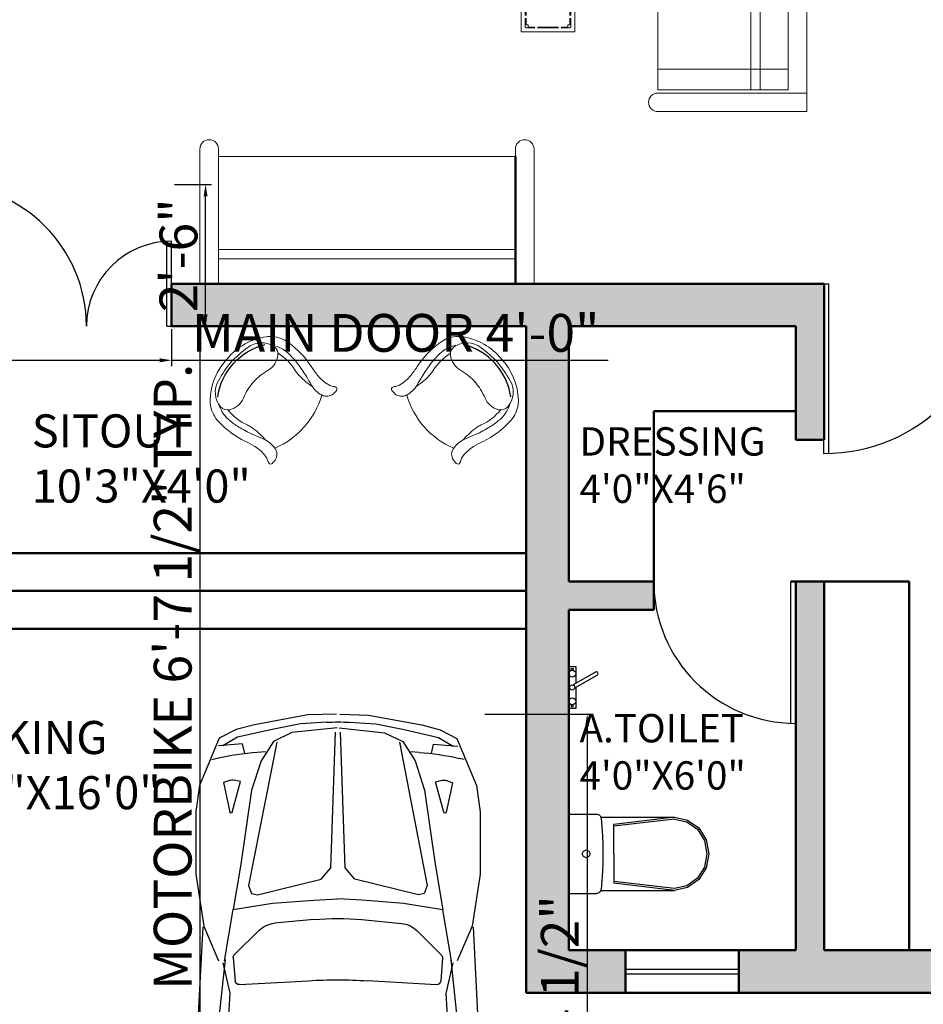
# Model space of a CAD drawing. Units: inches. Extents: x 3008 to 4088, y 1255 to 2137.
# Tile 5 of 30: x 3119 to 3310, y 1462 to 1670. Entities that reach past the tile are written whole.
import ezdxf

# ---------------------------------------------------------------- set-up
doc = ezdxf.new("R2010")
doc.units = ezdxf.units.IN
for name, color, linetype, lineweight in [('A-ANNO-DIMS', 2, 'Continuous', 18), ('A-AREA-IDEN', 7, 'Continuous', 18), ('A-DOOR', 4, 'Continuous', 25), ('A-FLOR-FIXT', 8, 'Continuous', 18), ('A-FURN', 8, 'Continuous', 18), ('A-GLAZ', 4, 'Continuous', 25), ('A-WALL', 7, 'Continuous', 50), ('A-WALL-PATT', 8, 'Continuous', 13), ('C-SITE-VEHC', 9, 'Continuous', 13)]:
    doc.layers.add(name, color=color, linetype=linetype, lineweight=lineweight)
for name, color, linetype in [('IFF-FURN-DETAIL', 250, 'Continuous'), ('L9012X$0', 2, 'Continuous'), ('SANTEH', 7, 'Continuous')]:
    doc.layers.add(name, color=color, linetype=linetype)
doc.styles.get("Standard").update_dxf_attribs({"font": 'arial.ttf'})
doc.dimstyles.new('ISO-25', dxfattribs={"dimtxt": 8, "dimasz": 2.5, "dimexe": 1.25, "dimexo": 0.625, "dimtad": 1, "dimdec": 1, "dimlunit": 3, "dimtxsty": 'Standard', "dimcen": 2.5, "dimadec": 0, "dimazin": 0, "dimtfac": 1, "dimtdec": 1, "dimtmove": 0, "dimatfit": 3, "dimfxl": 1, "dimarcsym": 0})

# ---------------------------------------------------------------- blocks, each defined once
blk = doc.blocks.new('MD')
for p, q in [((1902.58, 1512.86), (1902.58, 1482.86)), ((1903.58, 1512.86), (1903.58, 1482.86)), ((1949.58, 1482.86), (1949.58, 1500.86)), ((1950.58, 1482.86), (1950.58, 1500.86)), ((1902.58, 1482.86), (1903.58, 1482.86)), ((1949.58, 1482.86), (1950.58, 1482.86))]:
    blk.add_line(p, q)
for centre, radius, start, end in [((1902.58, 1482.86), 30, 0, 90), ((1950.58, 1482.86), 18, 90, 180)]:
    blk.add_arc(centre, radius, start, end)
blk = doc.blocks.new('A1099DC')
at = {"color": 0, "linetype": 'ByBlock'}
for p, q in [((1279.298465, 804.448389), (2201.430588, 851.890505)), ((2602.736326, 846.078152), (3356.693814, 785.353187)), ((3488.458929, 772.663345), (3732.658862, 759.86454)), ((272.228253, 749.073842), (265.114727, 718.465169)), ((1475.52921, 670.226262), (2282.402739, 758.004075)), ((2519.280414, 756.817792), (3387.476361, 653.818028)), ((2851.341839, 715.213377), (3126.60716, 755.701993)), ((139.051458, 595.027331), (190.951238, 683.213377)), ((179.200345, 564.515703), (190.951238, 709.631982)), ((398.733388, 644.315148), (411.280494, 678.748261)), ((411.280494, 678.748261), (588.616917, 641.417897)), ((1482.852352, 674.283145), (1175.286956, 622.180789)), ((1494.603245, 682.841284), (1678.210958, 641.166865)), ((1678.210958, 641.166865), (2462.684993, 690.847736)), ((2656.476214, 692.831247), (3376.704709, 662.004075)), ((3376.704709, 662.004075), (3510.708679, 626.736433)), ((3909.27561, 688.812956), (3837.725727, 693.401722)), ((3867.794139, 700.329656), (3900.059395, 686.767505)), ((3921.162781, 527.618662), (3921.162781, 676.138994)), ((3925.383812, 676.122818), (3955.306409, 663.545364)), ((92.537504, 388.14361), (139.051458, 595.027331)), ((405.405047, 577.538958), (396.874865, 615.894428)), ((589.014326, 626.599587), (405.405047, 577.538958)), ((1300.814287, 466.658131), (1445.712032, 613.104998)), ((1465.665584, 620.56924), (1602.893878, 610.287296)), ((236.043912, 551.980927), (179.200345, 564.515703)), ((1626.354615, 583.507504), (1602.652901, 169.222264)), ((3704.596898, 536.993674), (3795.675135, 473.385795)), ((229.117398, 477.634662), (225.714299, 427.957563)), ((1933.148906, 509.557888), (2330.980062, 522.200075)), ((3522.252709, 492.345257), (3666.066199, 475.644444)), ((3841.786866, 503.451367), (3910.58243, 515.096797)), ((3901.001848, 514.780764), (3957.150905, 375.772812)), ((1860.238743, -448.635916), (1859.369151, 433.397797)), ((2409.60024, 445.938054), (2410.49349, -460.09121)), ((3493.960271, 465.734554), (3507.923021, 209.166865)), ((3839.396146, 426.841284), (3888.358202, 417.538958)), ((3888.358202, 417.538958), (3983.199613, 359.957848)), ((57.774444, 216.608726), (92.537504, 388.14361)), ((1235.045743, 136.116317), (1257.419842, 373.755108)), ((3753.293176, 397.789551), (3815.226005, 132.124765)), ((3857.610793, 379.525702), (3912.067615, 118.157673)), ((3983.199613, 359.957848), (4035.448301, 43.94997)), ((49.168662, 58.00681), (57.774444, 216.608726)), ((3507.923021, 209.166865), (3507.64153, -4.333678)), ((4019.086894, 150.376168), (4084.69605, 122.469191)), ((4084.69605, 122.469191), (4109.177079, 60.329656)), ((4109.177079, 60.329656), (4113.094043, -5.158716)), ((3508.347273, -221.154823), (3507.644805, -7.65525)), ((3983.920268, -371.008369), (4035.545755, -54.898082)), ((4109.306686, -71.132359), (4113.094514, -5.636391)), ((49.301278, -76.507426), (58.219773, -235.092064)), ((4084.948231, -133.320044), (4109.306686, -71.132359)), ((1235.330373, -152.586046), (1258.173002, -390.180259)), ((3754.088875, -409.293325), (3815.497749, -143.506937)), ((3858.370276, -390.823819), (3912.311631, -129.348921)), ((4019.394229, -161.356334), (4084.948231, -133.320044)), ((58.219773, -235.092064), (93.320996, -406.558069)), ((1627.520644, -599.204785), (1603.002095, -184.967086)), ((3494.890446, -477.749545), (3508.347273, -221.154823)), ((93.320996, -406.558069), (140.24279, -613.349673)), ((3889.19258, -428.776374), (3983.920268, -371.008369)), ((3902.027941, -525.993061), (3957.902795, -386.874665)), ((230.077082, -495.779641), (226.576036, -446.109349)), ((3840.248961, -438.175225), (3889.19258, -428.776374)), ((1301.750547, -482.997536), (1446.936772, -629.158411)), ((1934.168526, -524.650381), (2332.023837, -536.508105)), ((3523.2353, -504.304409), (3667.01558, -487.320059)), ((3705.667171, -548.593196), (3796.61981, -484.805853)), ((3842.790735, -514.780444), (3911.609128, -526.290202)), ((237.150178, -570.112104), (180.331436, -582.758939)), ((180.331436, -582.758939), (192.368445, -727.851766)), ((3922.214148, -538.79118), (3922.506998, -687.311224)), ((140.24279, -613.349673), (192.316354, -701.433212)), ((406.561378, -595.336142), (398.106841, -633.708356)), ((590.267037, -644.034637), (406.561378, -595.336142)), ((1484.19765, -690.263206), (1176.530118, -638.767405)), ((1466.905004, -636.583294), (1604.112757, -626.030785)), ((3378.022114, -674.249887), (3511.956283, -638.718087)), ((400.0214, -662.125356), (412.636377, -696.533662)), ((412.636377, -696.533662), (589.898847, -658.853701)), ((1476.866524, -686.22077), (2283.911563, -772.40743)), ((1495.965396, -698.798158), (1679.490579, -656.761786)), ((1679.490579, -656.761786), (2464.061049, -704.895745)), ((2520.786439, -770.754078), (3388.777604, -666.042617)), ((2657.855804, -706.497136), (3378.022114, -674.249887)), ((3910.644841, -700.0086), (3839.104145, -704.738438)), ((3869.186159, -711.60707), (3901.424611, -697.981326)), ((3926.727989, -687.286725), (3956.625729, -674.650294)), ((273.723073, -767.133288), (266.549207, -736.538701)), ((2852.765183, -728.494989), (3128.109803, -768.440762)), ((1280.900818, -820.829563), (2203.124693, -866.453338)), ((2604.418191, -859.849707), (3358.254477, -797.638217)), ((3489.994314, -784.688586), (3734.168535, -771.408296))]:
    blk.add_line(p, q, dxfattribs=at)
for points in [[(-0.000783, 0.794772), (5.385043, 172.701749), (63.649891, 493.818028), (92.537504, 603.957563), (144.437284, 705.166865), (428.417214, 824.236633), (585.095796, 846.190121), (961.406447, 846.190121), (1274.27399, 797.818028), (1482.852352, 709.631982)], [(83.345007, -3.206171), (111.32237, 268.957533), (164.563706, 379.583828), (279.999271, 453.709838), (456.549665, 511.628518), (901.254996, 574.918954), (1175.286956, 622.180789), (1137.52997, 385.548359), (1118.345181, 137.317882), (1109.829198, -8.358455)], [(168.178729, 359.003083), (1030.214866, 528.397865), (1077.798844, 510.531569), (1086.170082, 475.285426), (992.832238, 91.960378), (924.218938, 35.478085), (108.447994, 6.034416)], [(0.019119, -19.392451), (5.743899, -191.288474), (64.641806, -512.289243), (93.746535, -622.371603), (145.845778, -723.478374), (430.059935, -841.987962), (586.7815, -863.632471), (963.091723, -863.198028), (1275.863278, -814.209121), (1484.26735, -725.611974)], [(83.356858, -15.227176), (111.870816, -287.335185), (165.330179, -397.856284), (280.911681, -471.754535), (457.575935, -529.324983), (902.4055, -592.045995), (1176.530118, -638.767405), (1138.306616, -402.209884), (1118.632407, -154.017717), (1109.829198, -8.358455)], [(168.904615, -377.268451), (1031.273389, -545.270714), (1078.822046, -527.310627), (1087.123771, -492.048047), (993.030273, -108.907787), (924.305735, -52.560894), (108.478017, -24.418246)]]:
    blk.add_lwpolyline(points, dxfattribs=at)
for centre, radius, start, end in [((2358.037832, -2192.08357), 3048, 85.395244, 92.945173), ((2399.99649, 588.663508), 206.166238, 54.649181, 124.776949), ((3392.740754, -1053.630025), 1828.8, 86.999806, 98.367602), ((1749.553982, 373.478072), 1524, 166.916578, 176.08111), ((3718.678317, 475.802507), 284.405862, 57.329946, 87.182375), ((2578.271641, -1134.295865), 1828.8, 87.549126, 93.623712), ((4191.049821, 605.937201), 363.988953, 166.096081, 196.353514), ((3908.462781, 676.138994), 12.7, 0, 86.330429), ((3896.252417, 523.051998), 152.4, 46.38363, 67.20138), ((446.46332, 626.922805), 50.8, 159.97873, 192.538409), ((587.047263, 633.961317), 7.62, 284.960009, 78.112462), ((1463.767788, 595.240237), 25.4, 85.715073, 135.304647), ((1600.996082, 584.958293), 25.4, 356.725615, 85.715073), ((3355.555414, 37.211519), 609.6, 55.070043, 75.255062), ((3320.85101, 50.338397), 847.430844, 356.245089, 44.519453), ((3700.933354, 318.064082), 435.542335, 30.457681, 46.38363), ((3204.184594, 25.950693), 1011.814461, 358.069446, 30.457681), ((1935.569151, 433.396333), 76.2, 91.82012, 179.9989), ((2333.400307, 446.03852), 76.2, 359.924458, 91.82012), ((3519.322741, 467.114813), 25.4, 83.37601, 183.115039), ((3654.346327, 374.722669), 101.6, 13.122645, 83.37601), ((3908.462781, 527.618662), 12.7, 279.607718, 0), ((1409.148822, 359.469565), 152.4, 135.304647, 174.62136), ((3708.414764, 348.440256), 152.4, 11.769371, 55.070043), ((2752.335538, -6.739118), 1524, 174.62136, 185.491615), ((4645.676894, -4.872483), 3048, 176.725615, 183.38736), ((3221.54491, -6.276527), 609.6, 346.99033, 13.122645), ((3315.283499, -6.18411), 609.6, 348.343604, 11.769371), ((1266.577845, -8.050136), 1219.2, 176.894161, 183.218814), ((3734.73098, -5.770579), 304.8, 350.724636, 9.388339), ((3320.962449, -62.69553), 847.430844, 315.593523, 3.867886), ((3204.248172, -38.537915), 1011.814461, 329.655294, 2.043529), ((1409.873518, -375.595566), 152.4, 185.491615, 224.808328), ((3655.096735, -386.42159), 101.6, 276.736965, 346.99033), ((3709.113243, -360.032616), 152.4, 305.042932, 348.343604), ((1936.438592, -448.484202), 76.2, 180.114076, 268.292856), ((2334.293902, -460.341926), 76.2, 268.292856, 0.188517), ((1750.305335, -388.625277), 1524, 184.031865, 193.196397), ((3520.255588, -479.079792), 25.4, 176.997936, 276.736965), ((4192.255091, -616.577407), 363.988953, 163.759461, 194.016894), ((3909.514173, -538.816222), 12.7, 0.112975, 80.505257), ((3355.640902, -49.500248), 609.6, 284.857913, 305.042932), ((3701.571953, -329.671253), 435.542335, 313.729345, 329.655294), ((447.716945, -644.638934), 50.8, 167.574566, 200.134245), ((588.314493, -651.400231), 7.62, 282.000513, 75.152966), ((1464.957267, -611.258083), 25.4, 224.808328, 274.397903), ((1602.165021, -600.705574), 25.4, 274.397903, 3.38736), ((3897.294828, -534.273643), 152.4, 292.911596, 313.729345), ((2576.048678, 1120.472221), 1828.8, 266.489263, 272.563849), ((3909.807023, -687.336265), 12.7, 273.782546, 0.112975), ((3390.675263, 1041.412497), 1828.8, 261.745373, 273.113169), ((3719.627907, -487.374382), 284.405862, 272.930601, 302.78303), ((2401.171182, -602.835323), 206.166238, 235.336026, 305.463794), ((2353.729565, 2177.823616), 3048, 267.167802, 274.717731)]:
    blk.add_arc(centre, radius, start, end, dxfattribs=at)
blk = doc.blocks.new('VI')
at = {"layer": 'L9012X$0'}
blk.add_blockref('A1099DC', (0, 0), dxfattribs=at)
blk = doc.blocks.new('D1')
for p, q in [((1805.96, 1500.36), (1805.96, 1464.36)), ((1806.96, 1500.36), (1806.96, 1464.36)), ((1805.96, 1464.36), (1806.96, 1464.36))]:
    blk.add_line(p, q)
blk.add_arc((1805.96, 1464.36), 36, 0, 90)
blk = doc.blocks.new('D2')
for p, q in [((1722.5, 1505.46), (1722.5, 1475.46)), ((1723.5, 1505.46), (1723.5, 1475.46)), ((1722.5, 1475.46), (1723.5, 1475.46))]:
    blk.add_line(p, q)
blk.add_arc((1722.5, 1475.46), 30, 0, 90)
blk = doc.blocks.new('WC 2 Symb_109')
at = {"layer": 'SANTEH'}
for p, q in [((0, 0), (0, 380)), ((0, 380), (132.4, 380)), ((153.6, 364.9), (506.8, 364.9)), ((506.3, 364.9), (215.7, 330.9)), ((506.3, 356), (215.7, 322)), ((215.7, 190), (215.7, 330.9)), ((215.7, 190), (215.7, 49.1)), ((506.3, 24), (215.7, 58)), ((506.3, 15.1), (215.7, 49.1)), ((153.8, 15.1), (506.8, 15.1)), ((0, 0), (132.4, 0))]:
    blk.add_line(p, q, dxfattribs=at)
for points in [[(154.6, 360.1), (153.9, 364.1), (152.3, 367.9), (150.2, 371.3), (147.4, 374.3), (144.1, 376.7), (140.5, 378.5), (136.5, 379.6), (132.4, 380)], [(154.6, 19.7), (158.6, 62.1), (161.4, 104.7), (163.1, 147.3), (163.7, 189.9), (163.1, 232.5), (161.4, 275.1), (158.6, 317.7), (154.6, 360.1)], [(506.3, 24), (565.5, 36.6), (615.7, 72.6), (649.2, 126.5), (661, 190), (649.2, 253.5), (615.7, 307.4), (565.5, 343.4), (506.3, 356)], [(506.8, 15.1), (569.2, 28.4), (622.2, 66.3), (657.6, 123.1), (670, 190), (657.6, 256.9), (622.2, 313.7), (569.2, 351.6), (506.8, 364.9)], [(132.4, 0), (136.5, 0.4), (140.4, 1.5), (144.1, 3.2), (147.3, 5.6), (150.1, 8.6), (152.3, 12), (153.8, 15.7), (154.6, 19.7)]]:
    blk.add_lwpolyline(points, dxfattribs=at)
blk.add_lwpolyline([(83.6, 208.5), (70.4, 203.1), (64.9, 190), (70.4, 176.9), (83.6, 171.5), (96.8, 176.9), (102.2, 190), (96.8, 203.1)], close=True, dxfattribs=at)
blk = doc.blocks.new('Faucet - kit sink top')
at = {"layer": 'SANTEH'}
for p, q in [((-5.5, -0.75), (-5.5, -1.25)), ((-4.94278, -0.75), (-5.5, -0.75)), ((-5.5, -1.25), (-4.94278, -1.25)), ((-0.14775, -1.7441), (3.56698, -8.1782)), ((4.43301, -7.6782), (0.71828, -1.2441)), ((4.94278, -0.75), (5.5, -0.75)), ((5.5, -1.25), (4.94278, -1.25)), ((5.5, -0.75), (5.5, -1.25))]:
    blk.add_line(p, q, dxfattribs=at)
blk.add_lwpolyline([(-0.00587, -2), (-6, -2), (-6, 0), (6, 0), (6, -2), (1.15195, -2)], dxfattribs=at)
for centre, radius in [((-4, -1), 1), ((4, -1), 1), ((0, -1), 0.75)]:
    blk.add_circle(centre, radius, dxfattribs=at)
blk.add_arc((4, -7.9282), 0.5, 210, 30, dxfattribs=at)
blk = doc.blocks.new('TABLE-30A')
at = {"color": 0, "linetype": 'ByBlock'}
for p, q in [((0, 0), (0, 0.55)), ((0, 0.55), (1.5, 0.55)), ((0.051, 0.508), (0.042, 0.499)), ((0.072, 0.508), (0.051, 0.508)), ((0.072, 0.478), (0.072, 0.508)), ((0.072, 0.508), (0.14, 0.508)), ((1.331, 0.508), (0.169, 0.508)), ((1.428, 0.508), (1.36, 0.508)), ((1.428, 0.508), (1.428, 0.478)), ((1.449, 0.508), (1.428, 0.508)), ((1.458, 0.499), (1.449, 0.508)), ((1.5, 0.55), (1.5, 0)), ((0.042, 0.499), (0.042, 0.478)), ((0.042, 0.478), (0.072, 0.478)), ((0.042, 0.478), (0.042, 0.41)), ((0.051, 0.478), (0.051, 0.41)), ((0.072, 0.499), (0.14, 0.499)), ((1.331, 0.499), (0.169, 0.499)), ((1.428, 0.499), (1.36, 0.499)), ((1.428, 0.478), (1.458, 0.478)), ((1.449, 0.478), (1.449, 0.41)), ((1.458, 0.478), (1.458, 0.499)), ((1.458, 0.478), (1.458, 0.41)), ((0.042, 0.169), (0.042, 0.381)), ((0.051, 0.169), (0.051, 0.381)), ((1.449, 0.381), (1.449, 0.169)), ((1.458, 0.381), (1.458, 0.169)), ((0.042, 0.072), (0.042, 0.14)), ((0.051, 0.072), (0.051, 0.14)), ((1.449, 0.072), (1.449, 0.14)), ((1.458, 0.072), (1.458, 0.14)), ((1.5, 0), (0, 0)), ((0.042, 0.072), (0.042, 0.051)), ((0.072, 0.072), (0.042, 0.072)), ((0.042, 0.051), (0.051, 0.042)), ((0.051, 0.042), (0.072, 0.042)), ((0.072, 0.042), (0.072, 0.072)), ((0.072, 0.051), (0.14, 0.051)), ((0.072, 0.042), (0.14, 0.042)), ((0.169, 0.051), (1.331, 0.051)), ((0.169, 0.042), (1.331, 0.042)), ((1.428, 0.051), (1.36, 0.051)), ((1.428, 0.042), (1.36, 0.042)), ((1.428, 0.072), (1.428, 0.042)), ((1.458, 0.072), (1.428, 0.072)), ((1.428, 0.042), (1.449, 0.042)), ((1.449, 0.042), (1.458, 0.051)), ((1.458, 0.051), (1.458, 0.072))]:
    blk.add_line(p, q, dxfattribs=at)
blk = doc.blocks.new('ILNG95')
for points in [[(120, 307.8, -0.32971), (50.6, 383.9, -0.036099), (49.5, 421.7, -0.497733), (75, 439.3, -0.070621), (96.1, 428.8, 0.101868), (132.6, 413.5, 0.091794), (258.7, 412, 0.024114), (350.8, 432.5, -0.090294), (637.9, 457.7, -0.132412), (774.5, 407, -0.068618), (816.3, 367.6, -0.184346), (942.9, -0.4, 1.803905)], [(120, 307.8, 0.138132), (243.9, 312.8, 0.001085), (324.6, 339.3, -0.034227), (462.2, 374.6, -0.033255), (566.6, 386.7, -0.137428), (726.9, 350.3, -4.561553)], [(120, 307.8, 0.138132), (243.9, 312.8, 0.001085), (324.6, 339.3, -0.034227), (462.2, 374.6, -0.033255), (566.6, 386.7, -0.137428), (726.9, 350.3, -4.561553)], [(639.1, -0.4, 0.078302), (611.9, 161.3, -0.233633), (633, 315.1, -0.28763), (710.5, 349.3, -0.317923), (874.6, 193.2, -0.032882), (899.6, 0, 1.140397)], [(639.1, -0.4, 0.078302), (611.9, 161.3, -0.233633), (633, 315.1, -0.28763), (710.5, 349.3, -0.317923), (874.6, 193.2, -0.032882), (899.6, 0, 1.140397)], [(235.1, 307.5, 0.064243), (394.2, 306.7, 0.04414), (433.1, 315, -0.118032), (643, 328.5, -6.296816)], [(235.1, 307.5, 0.064243), (394.2, 306.7, 0.04414), (433.1, 315, -0.118032), (643, 328.5, -6.296816)], [(120, -307.8, 0.32971), (50.6, -383.9, 0.036099), (49.5, -421.7, 0.497733), (75, -439.3, 0.070621), (96.1, -428.8, -0.101868), (132.6, -413.5, -0.091794), (258.7, -412, -0.024114), (350.8, -432.5, 0.090294), (637.9, -457.7, 0.132412), (774.5, -407, 0.068618), (816.3, -367.6, 0.184346), (942.9, 0.4, -1.803905)], [(639.1, 0.4, -0.078302), (611.9, -161.3, 0.233633), (633, -315.1, 0.28763), (710.5, -349.3, 0.317923), (874.6, -193.2, 0.032882), (899.6, 0, -1.140397)], [(639.1, 0.4, -0.078302), (611.9, -161.3, 0.233633), (633, -315.1, 0.28763), (710.5, -349.3, 0.317923), (874.6, -193.2, 0.032882), (899.6, 0, -1.140397)], [(120, -307.8, -0.138132), (243.9, -312.8, -0.001085), (324.6, -339.3, 0.034227), (462.2, -374.6, 0.033255), (566.6, -386.7, 0.137428), (726.9, -350.3, 4.561553)], [(120, -307.8, -0.138132), (243.9, -312.8, -0.001085), (324.6, -339.3, 0.034227), (462.2, -374.6, 0.033255), (566.6, -386.7, 0.137428), (726.9, -350.3, 4.561553)], [(235.1, -307.5, -0.064243), (394.2, -306.7, -0.04414), (433.1, -315, 0.118032), (643, -328.5, 6.296816)], [(235.1, -307.5, -0.064243), (394.2, -306.7, -0.04414), (433.1, -315, 0.118032), (643, -328.5, 6.296816)]]:
    blk.add_lwpolyline(points, format="xyb")
blk.add_arc((758.7, 0.8), 708.7, 154.32815, 205.80105)
at = {"layer": 'IFF-FURN-DETAIL'}
blk.add_arc((326.4, -1.7), 549.3, 326.8997, 34.66912, dxfattribs=at)
blk.add_arc((326.4, -1.7), 549.3, 326.8997, 34.66912, dxfattribs=at)
blk = doc.blocks.new('SOFA-L')
for p, q in [((35.53, 102.74), (67.02, 102.74)), ((67.02, 102.74), (67.02, 0.37)), ((0.3, 98.14), (0.3, 71.24)), ((63.09, 98.14), (0.3, 98.14)), ((35.53, 98.8), (63.09, 98.8)), ((35.53, 4.97), (35.53, 98.14)), ((63.09, 98.8), (63.09, 4.97)), ((0.3, 92.9), (57.18, 92.9)), ((57.18, 92.9), (57.18, 4.97)), ((0.3, 90.93), (55.21, 90.93)), ((55.21, 90.93), (55.21, 4.97)), ((63.09, 71.24), (0.3, 71.24)), ((40.78, 71.24), (0.3, 71.24)), ((63.09, 48.93), (35.53, 48.93)), ((63.09, 27.28), (35.53, 27.28)), ((63.09, 9.36), (35.53, 9.36)), ((63.09, 4.97), (35.53, 4.97)), ((67.02, 4.31), (35.53, 4.31)), ((67.02, 0.37), (35.53, 0.37))]:
    blk.add_line(p, q)
for centre in [(35.53, 100.77), (35.53, 2.34)]:
    blk.add_arc(centre, 1.97, 90, 270)
blk = doc.blocks.new('*D43')
at = {"layer": 'A-ANNO-DIMS', "color": 0, "lineweight": -2, "transparency": 16777216}
for p, q in [((3102.67, 1604.34), (3102.67, 1596.52)), ((3150.67, 1604.34), (3150.67, 1596.52)), ((3105.17, 1597.77), (3148.17, 1597.77)), ((3150.67, 1597.77), (3242.99, 1597.77))]:
    blk.add_line(p, q, dxfattribs=at)
at = {"layer": 'A-ANNO-DIMS', "color": 0, "transparency": 16777216}
for points in [[(3105.17, 1598.18), (3105.17, 1597.35), (3102.67, 1597.77)], [(3148.17, 1598.18), (3148.17, 1597.35), (3150.67, 1597.77)]]:
    blk.add_solid(points, dxfattribs=at)
at = {"layer": 'Defpoints', "color": 0, "transparency": 16777216}
for p in [(3102.67, 1604.97), (3150.67, 1604.97), (3150.67, 1597.77)]:
    blk.add_point(p, dxfattribs=at)
at = {"layer": 'A-ANNO-DIMS', "color": 0, "transparency": 16777216, "insert": (3198.08, 1602.53), "char_height": 8, "attachment_point": 5}
blk.add_mtext('MAIN DOOR 4\'-0"', dxfattribs=at)
blk = doc.blocks.new('*D44')
at = {"layer": 'A-ANNO-DIMS', "color": 0, "lineweight": -2, "transparency": 16777216}
for p, q in [((3151.29, 1634.97), (3159.12, 1634.97)), ((3157.87, 1607.47), (3157.87, 1632.47)), ((3151.29, 1604.97), (3159.12, 1604.97))]:
    blk.add_line(p, q, dxfattribs=at)
at = {"layer": 'A-ANNO-DIMS', "color": 0, "transparency": 16777216}
for points in [[(3157.45, 1632.47), (3158.28, 1632.47), (3157.87, 1634.97)], [(3157.45, 1607.47), (3158.28, 1607.47), (3157.87, 1604.97)]]:
    blk.add_solid(points, dxfattribs=at)
at = {"layer": 'Defpoints', "color": 0, "transparency": 16777216}
for p in [(3150.67, 1634.97), (3157.87, 1634.97), (3150.67, 1604.97)]:
    blk.add_point(p, dxfattribs=at)
at = {"layer": 'A-ANNO-DIMS', "color": 0, "transparency": 16777216, "insert": (3153.16, 1619.97), "char_height": 8, "attachment_point": 5, "rotation": 90}
blk.add_mtext('2\'-6"', dxfattribs=at)
blk = doc.blocks.new('*D61')
at = {"layer": 'A-ANNO-DIMS', "color": 0, "lineweight": -2, "transparency": 16777216}
for p, q in [((3156.71, 1459.08), (3156.71, 1600.04)), ((3145.38, 1459.08), (3157.96, 1459.08)), ((3156.71, 1381.91), (3156.71, 1456.58)), ((3145.38, 1379.41), (3157.96, 1379.41))]:
    blk.add_line(p, q, dxfattribs=at)
at = {"layer": 'A-ANNO-DIMS', "color": 0, "transparency": 16777216}
for points in [[(3156.29, 1456.58), (3157.12, 1456.58), (3156.71, 1459.08)], [(3156.29, 1381.91), (3157.12, 1381.91), (3156.71, 1379.41)]]:
    blk.add_solid(points, dxfattribs=at)
at = {"layer": 'Defpoints', "color": 0, "transparency": 16777216}
for p in [(3144.76, 1459.08), (3156.71, 1459.08), (3144.76, 1379.41)]:
    blk.add_point(p, dxfattribs=at)
at = {"layer": 'A-ANNO-DIMS', "color": 0, "transparency": 16777216, "insert": (3151.94, 1530.81), "char_height": 8, "attachment_point": 5, "rotation": 90}
blk.add_mtext('MOTORBIKE 6\'-7 1/2" TYP.', dxfattribs=at)
blk = doc.blocks.new('*D63')
at = {"layer": 'A-ANNO-DIMS', "color": 0, "lineweight": -2, "transparency": 16777216}
for p, q in [((3216.92, 1522.92), (3239.83, 1522.92)), ((3238.58, 1520.42), (3238.58, 1376.84)), ((3216.92, 1374.34), (3239.83, 1374.34))]:
    blk.add_line(p, q, dxfattribs=at)
at = {"layer": 'A-ANNO-DIMS', "color": 0, "transparency": 16777216}
for points in [[(3238.16, 1520.42), (3238.99, 1520.42), (3238.58, 1522.92)], [(3238.16, 1376.84), (3238.99, 1376.84), (3238.58, 1374.34)]]:
    blk.add_solid(points, dxfattribs=at)
at = {"layer": 'Defpoints', "color": 0, "transparency": 16777216}
for p in [(3216.29, 1522.92), (3216.29, 1374.34), (3238.58, 1374.34)]:
    blk.add_point(p, dxfattribs=at)
at = {"layer": 'A-ANNO-DIMS', "color": 0, "transparency": 16777216, "insert": (3233.82, 1448.63), "char_height": 8, "attachment_point": 5, "rotation": 90}
blk.add_mtext('CAR 12\'-4 1/2"', dxfattribs=at)

msp = doc.modelspace()

# ---------------------------------------------------------------- hatches: boundary and pattern name
at = {"layer": 'A-WALL-PATT'}
h = msp.add_hatch(color=256, dxfattribs=at)
h.dxf.hatch_style = 1
h.paths.add_polyline_path([(3102.67, 1625.97), (3093.67, 1625.97), (3093.67, 1540.97), (3102.67, 1540.97)])
h.paths.add_polyline_path([(3102.67, 1784.97), (3252.67, 1784.97), (3252.67, 1790.97), (3102.67, 1790.97), (3102.67, 1892.97), (3093.67, 1892.97), (3093.67, 1667.97), (3102.67, 1667.97)])
h.paths.add_polyline_path([(3192.67, 1943.97), (3093.67, 1943.97), (3093.67, 1934.97), (3102.67, 1934.97), (3192.67, 1934.97)])
h.paths.add_polyline_path([(3264.67, 1943.97), (3234.67, 1943.97), (3234.67, 1934.97), (3246.67, 1934.97), (3246.67, 1868.97), (3252.67, 1868.97), (3252.67, 1934.97), (3264.67, 1934.97)])
h.paths.add_polyline_path([(3330.67, 1943.97), (3288.67, 1943.97), (3288.67, 1934.97), (3300.67, 1934.97), (3300.67, 1838.97), (3246.67, 1838.97), (3246.67, 1826.97), (3252.67, 1826.97), (3252.67, 1832.97), (3306.67, 1832.97), (3306.67, 1934.97), (3330.67, 1934.97)])
h.paths.add_polyline_path([(3390.67, 1943.97), (3360.67, 1943.97), (3360.67, 1934.97), (3390.67, 1934.97)])
h.paths.add_polyline_path([(3465.67, 1943.97), (3432.67, 1943.97), (3432.67, 1934.97), (3456.67, 1934.97), (3456.67, 1883.97), (3465.67, 1883.97)])
h.paths.add_polyline_path([(3465.67, 1841.97), (3456.67, 1841.97), (3456.67, 1790.97), (3370.67, 1790.97), (3370.67, 1784.97), (3456.67, 1784.97), (3456.67, 1759.47), (3465.67, 1759.47)])
h.paths.add_polyline_path([(3465.67, 1693.47), (3456.67, 1693.47), (3456.67, 1667.97), (3330.67, 1667.97), (3330.67, 1643.97), (3336.67, 1643.97), (3336.67, 1661.97), (3456.67, 1661.97), (3456.67, 1649.97), (3465.67, 1649.97)])
h.paths.add_polyline_path([(3465.67, 1625.97), (3456.67, 1625.97), (3456.67, 1613.97), (3324.67, 1613.97), (3324.67, 1604.97), (3456.67, 1604.97), (3456.67, 1571.97), (3465.67, 1571.97)])
h.paths.add_polyline_path([(3465.67, 1505.97), (3456.67, 1505.97), (3456.67, 1472.97), (3438.67, 1472.97), (3438.67, 1463.97), (3465.67, 1463.97)])
h.paths.add_polyline_path([(3396.67, 1472.97), (3354.67, 1472.97), (3354.67, 1463.97), (3396.67, 1463.97)])
h.paths.add_polyline_path([(3312.67, 1472.97), (3288.67, 1472.97), (3288.67, 1550.97), (3282.67, 1550.97), (3282.67, 1472.97), (3270.67, 1472.97), (3270.67, 1463.97), (3312.67, 1463.97)])
h.paths.add_polyline_path([(3246.67, 1472.97), (3234.67, 1472.97), (3234.67, 1544.97), (3252.67, 1544.97), (3252.67, 1550.97), (3234.67, 1550.97), (3234.67, 1604.97), (3282.67, 1604.97), (3282.67, 1580.97), (3288.67, 1580.97), (3288.67, 1613.97), (3150.67, 1613.97), (3150.67, 1604.97), (3225.67, 1604.97), (3225.67, 1463.97), (3246.67, 1463.97)])

# ---------------------------------------------------------------- linework, layer by layer
at = {"layer": 'A-FURN'}
for p, q in [((3156.67, 1613.97), (3156.67, 1642.46)), ((3160.6, 1613.97), (3160.6, 1642.46)), ((3223.39, 1613.97), (3223.39, 1642.46)), ((3227.33, 1613.97), (3227.33, 1642.46)), ((3223.39, 1640.87), (3160.6, 1640.87)), ((3160.6, 1613.97), (3160.6, 1640.87)), ((3160.6, 1621.18), (3223.39, 1621.18)), ((3160.6, 1619.21), (3223.39, 1619.21)), ((3227.33, 1613.97), (3156.67, 1613.97))]:
    msp.add_line(p, q, dxfattribs=at)
for centre in [(3158.63, 1642.46), (3225.36, 1642.46)]:
    msp.add_arc(centre, 1.97, 0, 180, dxfattribs=at)
at = {"layer": 'A-GLAZ'}
for p, q in [((3246.67, 1468.97), (3270.67, 1468.97)), ((3246.67, 1467.97), (3270.67, 1467.97))]:
    msp.add_line(p, q, dxfattribs=at)
at = {"layer": 'A-WALL'}
for p, q in [((3223.39, 1613.97), (3223.39, 1640.87)), ((3150.67, 1613.97), (3288.67, 1613.97)), ((3150.67, 1604.97), (3150.67, 1613.97)), ((3288.67, 1580.97), (3288.67, 1613.97)), ((3150.67, 1604.97), (3225.67, 1604.97)), ((3225.67, 1604.97), (3225.67, 1463.97)), ((3234.67, 1604.97), (3282.67, 1604.97)), ((3234.67, 1550.97), (3234.67, 1604.97)), ((3282.67, 1580.97), (3282.67, 1604.97)), ((3252.67, 1550.97), (3252.67, 1586.97)), ((3252.67, 1586.97), (3282.67, 1586.97)), ((3288.67, 1580.97), (3282.67, 1580.97)), ((3102.67, 1556.97), (3225.67, 1556.97)), ((3252.67, 1550.97), (3234.67, 1550.97)), ((3252.67, 1544.97), (3252.67, 1550.97)), ((3306.67, 1550.97), (3281.67, 1550.97)), ((3282.67, 1472.97), (3282.67, 1550.97)), ((3288.67, 1472.97), (3288.67, 1550.97)), ((3306.67, 1472.97), (3306.67, 1550.97)), ((3102.67, 1548.97), (3225.67, 1548.97)), ((3234.67, 1472.97), (3234.67, 1544.97)), ((3252.67, 1544.97), (3234.67, 1544.97)), ((3225.67, 1540.97), (3093.67, 1540.97)), ((3282.67, 1472.97), (3234.67, 1472.97)), ((3246.67, 1463.97), (3246.67, 1472.97)), ((3270.67, 1463.97), (3270.67, 1472.97)), ((3456.67, 1472.97), (3288.67, 1472.97)), ((3465.67, 1463.97), (3225.67, 1463.97))]:
    msp.add_line(p, q, dxfattribs=at)

# ---------------------------------------------------------------- block references
at = {"layer": 'A-DOOR'}
msp.add_blockref('MD', (1200.08, 122.1), dxfattribs=at)
at = {"layer": 'A-DOOR', "xscale": -1, "rotation": 180}
msp.add_blockref('D1', (1482.7, 3078.33), dxfattribs=at)
at = {"layer": 'A-DOOR', "rotation": 180}
msp.add_blockref('D2', (5005.16, 3026.42), dxfattribs=at)
at = {"layer": 'A-FLOR-FIXT'}
for name, p, xscale, yscale, zscale, rotation in [('Faucet - kit sink top', (3234.67, 1528.55), 0.7356136897818673, 0.7356136897818673, 0.7356136897818673, 90), ('WC 2 Symb_109', (3234.67, 1501.76), -0.0441898926459964, 0.0441898926459964, 0.0441898926459964, 180)]:
    msp.add_blockref(name, p, dxfattribs=dict(at, xscale=xscale, yscale=yscale, zscale=zscale, rotation=rotation))
at = {"layer": 'A-FURN'}
msp.add_blockref('SOFA-L', (3218, 1650), dxfattribs=at)
for name, p, xscale, yscale, zscale, rotation in [('TABLE-30A', (3224.59, 1698.28), 20.70834898381633, 20.70834898381633, 20.70834898381633, 270), ('ILNG95', (3179.66, 1582.87), -0.0243705291132055, 0.0243705291132055, 0.0243705291132055, 318.5881218623716), ('ILNG95', (3203.18, 1582.87), 0.0243705291132055, 0.0243705291132055, 0.0243705291132055, 41.41187813762839)]:
    msp.add_blockref(name, p, dxfattribs=dict(at, xscale=xscale, yscale=yscale, zscale=zscale, rotation=rotation))
at = {"layer": 'C-SITE-VEHC', "xscale": -0.0351896714874634, "yscale": 0.0351896714874634, "zscale": 0.0351896714874634, "rotation": 90}
msp.add_blockref('VI', (3185.57, 1522.92), dxfattribs=at)

# ---------------------------------------------------------------- texts
at = {"layer": 'A-AREA-IDEN', "attachment_point": 1}
for s, insert, char_height in [('{\\fTimes New Roman|b0|i0|c0|p18;SITOUT\\P10\'3"X4\'0"}', (3121.1, 1586.33), 7), ('{\\fTimes New Roman|b0|i0|c0|p18;DRESSING\\P4\'0"X4\'6"}', (3236.95, 1583.6), 6), ('{\\fTimes New Roman|b0|i0|c0|p18;A.TOILET\\P4\'0"X6\'0"}', (3236.95, 1522.94), 6), ('{\\fTimes New Roman|b0|i0|c0|p18;PARKING\\P15\'1"X16\'0"}', (3096.73, 1521.46), 7)]:
    msp.add_mtext_dynamic_manual_height_columns(s, width=105.6127, gutter_width=12.5, heights=[0], dxfattribs=dict(at, insert=insert, char_height=char_height))

# ---------------------------------------------------------------- dimensions: what is measured, and where the dimension line sits
at = {"layer": 'A-ANNO-DIMS'}
dim = msp.add_linear_dim(base=(3157.87, 1634.97), p1=(3150.67, 1604.97), p2=(3150.67, 1634.97), angle=90, dimstyle='ISO-25', override={"dimdec": 1, "dimrnd": 0, "dimzin": 1, "dimlunit": 4, "dimfrac": 2}, dxfattribs=at)
dim.commit()
dim.dimension.update_dxf_attribs({"geometry": '*D44', "text_midpoint": (3153.16, 1619.97)})
dim = msp.add_linear_dim(base=(3150.67, 1597.77), p1=(3102.67, 1604.97), p2=(3150.67, 1604.97), text='MAIN DOOR <>', dimstyle='ISO-25', override={"dimdec": 1, "dimrnd": 0, "dimzin": 1, "dimlunit": 4, "dimfrac": 2}, dxfattribs=at)
dim.commit()
dim.dimension.update_dxf_attribs({"geometry": '*D43', "text_midpoint": (3198.08, 1602.53)})
for base, p1, p2, angle, text, picture, middle in [((3156.71, 1459.08), (3144.76, 1379.41), (3144.76, 1459.08), 90, 'MOTORBIKE <> TYP.', '*D61', (3151.94, 1530.81)), ((3238.58, 1374.34), (3216.29, 1522.92), (3216.29, 1374.34), 270, 'CAR <>', '*D63', (3233.82, 1448.63))]:
    dim = msp.add_linear_dim(base=base, p1=p1, p2=p2, angle=angle, text=text, dimstyle='ISO-25', override={"dimdec": 1, "dimrnd": 0, "dimzin": 1, "dimlunit": 4, "dimfrac": 2}, dxfattribs=at)
    dim.commit()
    dim.dimension.update_dxf_attribs({"geometry": picture, "text_midpoint": middle})

doc.saveas('drawing.dxf')
